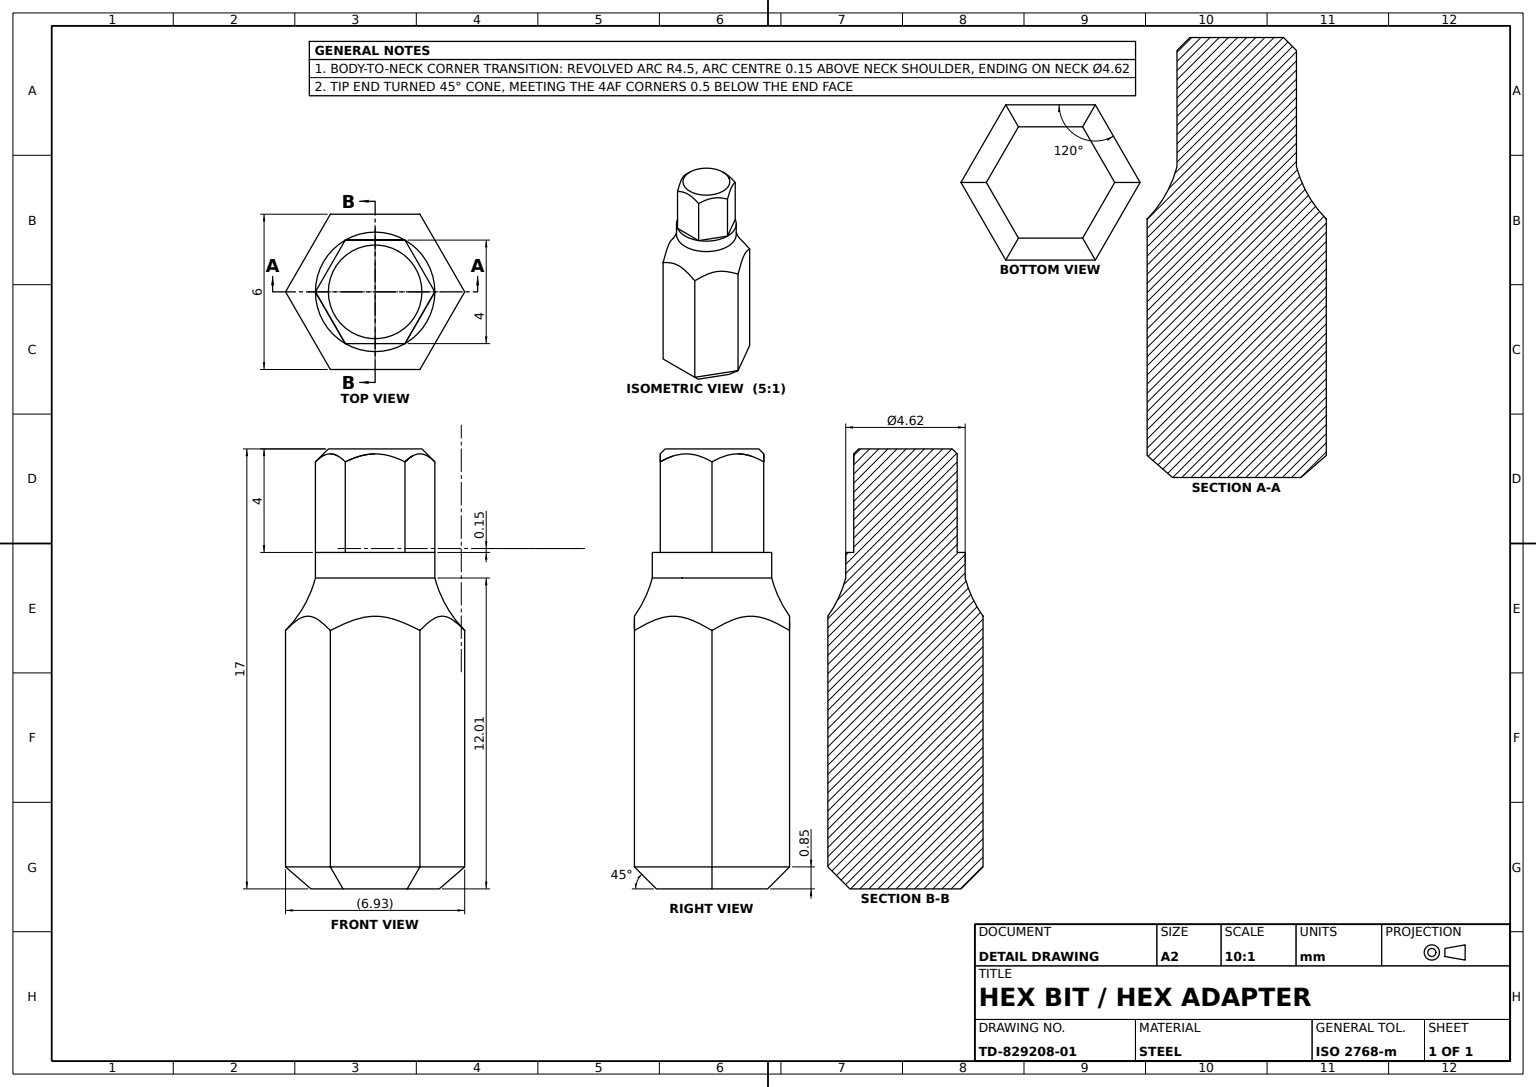
SolidWorks part; units mm, degrees
material "Plain Carbon Steel"
ref_plane "Front Plane" through (0, 0, 0) normal (0, 0, 1) x (1, 0, 0)
ref_plane "Top Plane" through (0, 0, 0) normal (0, 1, 0) x (1, 0, 0)
ref_plane "Right Plane" through (0, 0, 0) normal (1, 0, 0) x (0, 0, -1)
sketch "Hex Body Profile 6AF" plane through (0, 0, 0) normal (0, 1, 0) x (1, 0, 0)
  line L1 (3.4641, 0) -> (1.7321, 3)
  line L2 (1.7321, 3) -> (-1.7321, 3)
  line L3 (-1.7321, 3) -> (-3.4641, 0)
  line L4 (-3.4641, 0) -> (-1.7321, -3)
  line L5 (-1.7321, -3) -> (1.7321, -3)
  line L6 (1.7321, -3) -> (3.4641, 0)
  circle A0 centre (0, 0) radius 3 construction
  dimension "D1" = 6
extrude "Hex Body 6AF x17" add sketch "Hex Body Profile 6AF" along normal blind 17
chamfer "Edge Chamfer 0.85" distance 0.85 angle 45 6 edges at (2.5981, 0, -1.5) (0, 0, -3) (-2.5981, 0, -1.5) (-2.5981, 0, 1.5) (0, 0, 3) (2.5981, 0, 1.5)
sketch "Hex Tip Profile 4AF" plane through (0, 17, 0) normal (0, 1, 0) x (1, 0, 0)
  line L1 (2.3094, 0) -> (1.1547, 2)
  line L2 (1.1547, 2) -> (-1.1547, 2)
  line L3 (-1.1547, 2) -> (-2.3094, 0)
  line L4 (-2.3094, 0) -> (-1.1547, -2)
  line L5 (-1.1547, -2) -> (1.1547, -2)
  line L6 (1.1547, -2) -> (2.3094, 0)
  circle A0 centre (0, 0) radius 2 construction
  dimension "D1" = 4
extrude "Hex Tip 4AF x4" cut sketch "Hex Tip Profile 4AF" against normal blind 4 flip side to cut
sketch "Neck Groove Profile" plane through (0, 0, 0) normal (0, 0, 1) x (1, 0, 0)
  line L1 (0, 17) -> (0, 6.0282)
  line L2 (-1.1547, 17) -> (1.1547, 17) construction
  line L4 (3.4583, 9.9918) -> (3.4583, 12.012)
  line L7 (2.3094, 12.012) -> (3.4583, 12.012)
  line L12 (-3.4641, 12.012) -> (-3.4641, 13)
  line L14 (-3.4641, 13) -> (-2.3094, 13)
  arc A0 (2.3094, 12.012) -> (3.4583, 9.9918) centre (6.6629, 13.1511) ccw
  arc A2 (-3.4641, 12.012) -> (-2.3094, 13) centre (-3.3094, 13) ccw
  dimension "D1" = 4.5
  dimension "D2" = 1
  dimension "D3" = 0.1547
  dimension "D4" = 5.9838
  dimension "D5" = 5.7735
  dimension "D6" = 6.9224
  dimension "D7" = 10.127
revolve "Neck Groove" cut sketch "Neck Groove Profile" angle 360 about L1
sketch "Hex Corner Turn Profile" plane through (0, 0, 0) normal (0, 0, 1) x (1, 0, 0)
  line L3 (2.3094, 13) -> (2.3094, 17)
  line L4 (2.3094, 17) -> (2.3094, 12.012)
  line L5 (2.3094, 19.6763) -> (11.0924, 19.4735)
  line L6 (11.0924, 19.4735) -> (3.4583, 9.9918)
  line L7 (2.3094, 19.6763) -> (2.3094, 16.8377)
  line L8 (0, 0) -> (0, 28.5345)
  line L9 (1.2413, 0) -> (-1.2413, 0) construction
  arc A4 (2.3094, 12.012) -> (3.4583, 9.9918) centre (6.6629, 13.1511) ccw
  dimension "D1" = 4.5
  dimension "D2" = 2.3094
  dimension "D3" = 3.4583
  dimension "D4" = 6.6629
  dimension "D5" = 11.0924
  dimension "D6" = 9.9918
  dimension "D7" = 28.5345
  dimension "D8" = 13
  dimension "D10" = 16.8377
  dimension "D11" = 17
  dimension "D12" = 19.4735
  dimension "D13" = 19.6763
revolve "Hex Corner Turn" cut sketch "Hex Corner Turn Profile" angle 360 about L8
sketch "Tip Chamfer Profile" plane through (0, 0, 0) normal (0, 0, 1) x (1, 0, 0)
  line L0 (-1.8094, 17) -> (-2.3094, 17)
  line L3 (-2.3094, 16.5) -> (-1.8094, 17)
  line L4 (-2.3094, 16.5) -> (-2.3094, 17)
  line L6 (0, 17) -> (0, 14.2838)
  line L7 (-1.1547, 17) -> (1.1547, 17) construction
  dimension "D1" = 45
  dimension "D2" = 0.5
  dimension "D3" = 2.3094
  dimension "D4" = 2.7162
revolve "Tip Chamfer 0.5x45" cut sketch "Tip Chamfer Profile" angle 360 about L6
